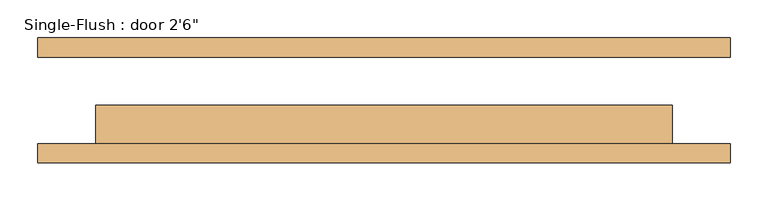
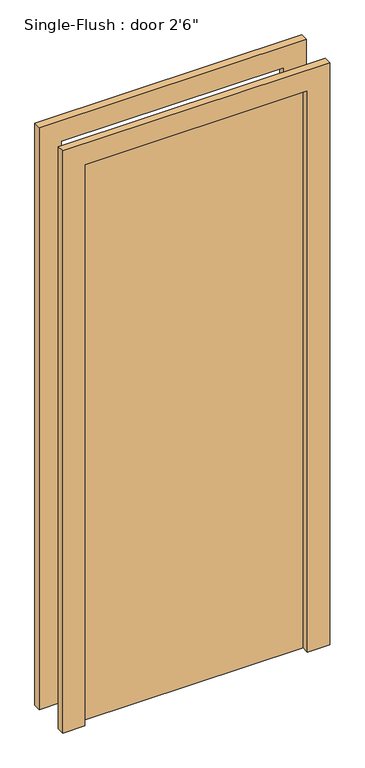
"""IFC4 building model written with IfcOpenShell, lengths in millimetres: door geometry."""

from ifc_helpers import new_model, si_unit, frame, origin, origin_with_axes, place, context, project, spatial, polyline, outline, extrude, source, transform, mapped, element, save


def door_f2b275c1(model_context):
    return source(origin(), model_context, "Body", "SweptSolid", [
        extrude(outline(polyline([(2108.2, -457.2), (0.0, -457.2), (0.0, -381.0), (2032.0, -381.0), (2032.0, 381.0), (0.0, 381.0), (0.0, 457.2), (2108.2, 457.2), (2108.2, -457.2)])), frame((0.0, -82.55, 0.0), z_axis=(0.0, 1.0, 0.0), x_axis=(0.0, 0.0, 1.0)), (0.0, 0.0, 1.0), 25.4),
        extrude(outline(polyline([(2108.2, 457.2), (2108.2, -457.2), (0.0, -457.2), (0.0, -381.0), (2032.0, -381.0), (2032.0, 381.0), (0.0, 381.0), (0.0, 457.2), (2108.2, 457.2)])), frame((0.0, 57.15, 0.0), z_axis=(0.0, 1.0, 0.0), x_axis=(0.0, 0.0, 1.0)), (0.0, 0.0, 1.0), 25.4),
        extrude(outline(polyline([(381.0, -6.35), (381.0, -57.15), (-381.0, -57.15), (-381.0, -6.35), (381.0, -6.35)])), origin_with_axes(), (0.0, 0.0, 1.0), 2032.0),
    ])


if __name__ == "__main__":
    model = new_model("IFC4")
    model_context = context("Model", 3, world=origin())
    ifc_project = project(units=[si_unit("LENGTHUNIT", "METRE", prefix="MILLI")], contexts=[model_context])
    site = spatial("IfcSite", under=ifc_project)
    building = spatial("IfcBuilding", under=site)
    placement = place(None, origin())
    door_shape = door_f2b275c1(model_context)
    element("IfcDoor", 1, ObjectType="Single-Flush : door 2'6\"", at=placement, inside=building, context=model_context, shape_type="MappedRepresentation", body=[
        mapped(door_shape, transform((0.0, 0.0, 0.0), x_axis=(1.0, 0.0, 0.0), y_axis=(0.0, 1.0, 0.0), z_axis=(0.0, 0.0, 1.0))),
    ])
    save(model, "model.ifc")

# Revit data of these elements
# Type "Single-Flush : door 2'6\""
#   Type Mark = "10"
#   Construction Type Id = "MDOOR"
#   Assembly Code = "C1020"
#   Analytic Construction = "Metal"
#   Thickness = 0' - 2"
#   Heat Transfer Coefficient (U) = 0.651978 BTU/(h·ft²·°F)
#   Height = 6' - 8"
#   Trim Projection Ext = 0' - 1"
#   Trim Projection Int = 0' - 1"
#   Trim Width = 0' - 3"
#   Width = 2' - 6"
#   Define Thermal Properties by = 1
#   Door Material = Door - Panel
#   Frame Material = Door - Frame
#   Visual Light Transmittance = 0
#   Solar Heat Gain Coefficient = 0
#   Function = (empty or 0)
#   Wall Closure = (empty or 0)
# Element 1 (IfcDoor, "Single-Flush : door 2'6\"")
#   Materials on its faces: "Door - Frame", "Door - Panel"
# Materials
#   "Door - Panel": class "Wood", colour RGB 210 159 95, transparency 0, Cost = 0
#   "Door - Frame": colour RGB 118 70 51, transparency 0, Cost = 0
